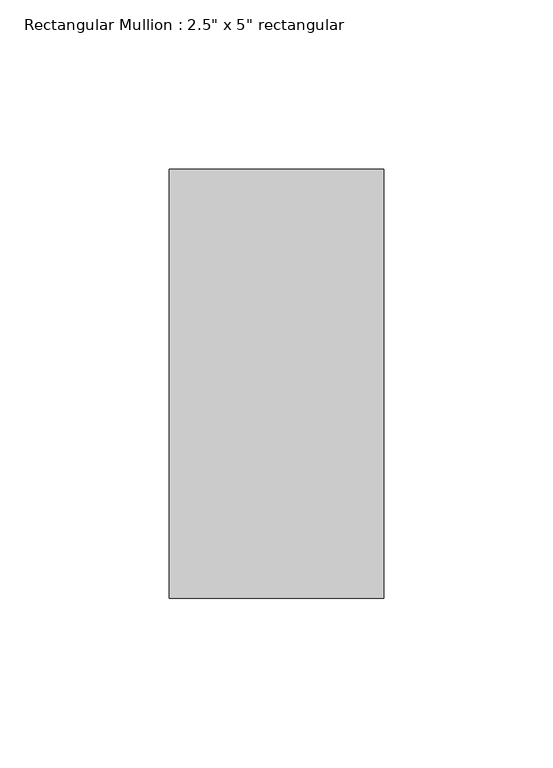
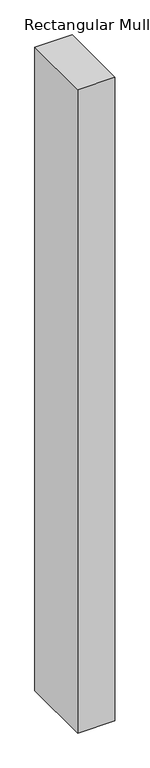
"""IFC4 building model written with IfcOpenShell, lengths in millimetres: member geometry."""

from ifc_helpers import new_model, si_unit, frame, origin, place, context, project, spatial, polyline, outline, extrude, source, transform, mapped, element, save


def member_f0038585(model_context):
    return source(origin(), model_context, "Body", "SweptSolid", [
        extrude(outline(polyline([(0.0, 63.5), (0.0, -63.5), (-63.5, -63.5), (-63.5, 63.5), (0.0, 63.5)])), frame((0.0, 0.0, -1164.1666667), z_axis=(0.0, 0.0, 1.0), x_axis=(1.0, 0.0, 0.0)), (0.0, 0.0, 1.0), 1164.1666667),
    ])


if __name__ == "__main__":
    model = new_model("IFC4")
    model_context = context("Model", 3, world=origin())
    ifc_project = project(units=[si_unit("LENGTHUNIT", "METRE", prefix="MILLI")], contexts=[model_context])
    site = spatial("IfcSite", under=ifc_project)
    building = spatial("IfcBuilding", under=site)
    placement = place(None, origin())
    member_shape = member_f0038585(model_context)
    element("IfcMember", 1, ObjectType="Rectangular Mullion : 2.5\" x 5\" rectangular", at=placement, inside=building, context=model_context, shape_type="MappedRepresentation", body=[
        mapped(member_shape, transform((0.0, 0.0, 0.0), x_axis=(1.0, 0.0, 0.0), y_axis=(0.0, 1.0, 0.0), z_axis=(0.0, 0.0, 1.0))),
    ])
    save(model, "model.ifc")

# Revit data of these elements
# Type "Rectangular Mullion : 2.5\" x 5\" rectangular"
#   built-in parameter 1007304 = 0.416667 (stored number, unit not read)
#   built-in parameter 1007301 = 0.104167 (stored number, unit not read)
#   built-in parameter 1007300 = 0.104167 (stored number, unit not read)
# Element 1 (IfcMember, "Rectangular Mullion : 2.5\" x 5\" rectangular")
#   Materials on its faces: "Aluminum"
# Materials
#   "Aluminum": class "Metal", colour RGB 247 247 247, transparency 0, Description = "Aluminum 6061", Cost = 0
